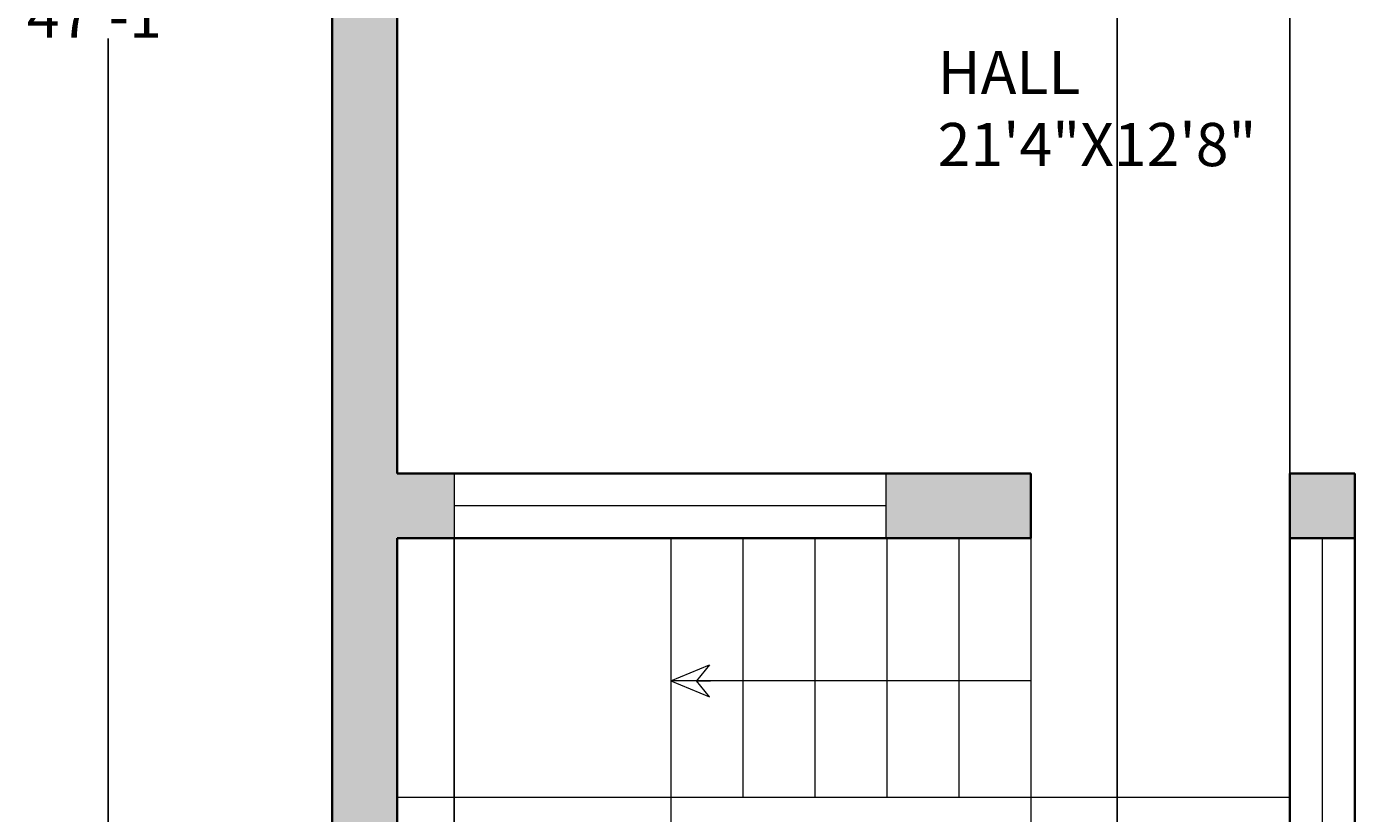
# Model space of a CAD drawing. Units: inches. Extents: x 37 to 706, y -568 to 110.
# Tile 7 of 24: x 37 to 223, y -342 to -233. Entities that reach past the tile are written whole.
import ezdxf

# ---------------------------------------------------------------- set-up
doc = ezdxf.new("R2010")
doc.units = ezdxf.units.IN
doc.header["$MEASUREMENT"] = 0
for name, color, linetype, lineweight in [('A-ANNO-DIMS', 2, 'Continuous', 18), ('A-AREA-IDEN', 7, 'Continuous', 18), ('A-FLOR-STRS', 7, 'Continuous', 18), ('A-GLAZ', 4, 'Continuous', 18), ('A-WALL', 7, 'Continuous', 35), ('A-WALL-PATT', 252, 'Continuous', 13)]:
    doc.layers.add(name, color=color, linetype=linetype, lineweight=lineweight)
doc.styles.get("Standard").update_dxf_attribs({"font": 'arial.ttf'})
doc.dimstyles.get("Standard").update_dxf_attribs({"dimtxt": 0.18, "dimasz": 0.18, "dimexe": 0.18, "dimexo": 0.0625, "dimgap": 0.09, "dimtad": 0, "dimtih": 1, "dimtoh": 1, "dimdec": 0, "dimzin": 0, "dimdsep": 46, "dimlunit": 3, "dimtxsty": 'Standard', "dimcen": 0.09, "dimadec": 0, "dimazin": 0, "dimtfac": 1, "dimtdec": 0, "dimtofl": 0, "dimtmove": 0, "dimatfit": 3, "dimfxl": 1, "dimtolj": 1, "dimtzin": 0, "dimarcsym": 0})

# ---------------------------------------------------------------- blocks, each defined once
blk = doc.blocks.new('*D3')
at = {"layer": 'A-ANNO-DIMS', "color": 0, "lineweight": -2, "transparency": 16777216}
for p, q in [((78.9, 51.29), (47.67, 51.29)), ((47.85, 51.11), (47.85, -228.11)), ((47.85, -513.53), (47.85, -234.31)), ((78.9, -513.71), (47.67, -513.71))]:
    blk.add_line(p, q, dxfattribs=at)
at = {"layer": 'A-ANNO-DIMS', "color": 0, "transparency": 16777216}
for points in [[(47.82, 51.11), (47.88, 51.11), (47.85, 51.29)], [(47.82, -513.53), (47.88, -513.53), (47.85, -513.71)]]:
    blk.add_solid(points, dxfattribs=at)
at = {"layer": 'Defpoints', "color": 0, "transparency": 16777216}
for p in [(78.96, 51.29), (47.85, -513.71), (78.96, -513.71)]:
    blk.add_point(p, dxfattribs=at)
at = {"layer": 'A-ANNO-DIMS', "color": 0, "transparency": 16777216, "insert": (47.85, -231.21), "char_height": 6, "attachment_point": 5}
blk.add_mtext('\\A1;47\'-1"', dxfattribs=at)
blk = doc.blocks.new('WIN-60')
for p, q in [((60, 9), (0, 9)), ((0, 9), (0, 0)), ((60, 0), (60, 9)), ((60, 4.5), (0, 4.5)), ((0, 0), (60, 0))]:
    blk.add_line(p, q)
blk = doc.blocks.new('*D51')
at = {"layer": 'A-ANNO-DIMS', "color": 0, "lineweight": -2, "transparency": 16777216}
for p, q in [((220.96, -294.77), (220.96, -567.64)), ((251.96, -294.77), (251.96, -567.64)), ((221.14, -567.46), (236.13, -567.46)), ((251.78, -567.46), (236.79, -567.46))]:
    blk.add_line(p, q, dxfattribs=at)
at = {"layer": 'A-ANNO-DIMS', "color": 0, "transparency": 16777216}
for points in [[(221.14, -567.43), (221.14, -567.49), (220.96, -567.46)], [(251.78, -567.43), (251.78, -567.49), (251.96, -567.46)]]:
    blk.add_solid(points, dxfattribs=at)
at = {"layer": 'Defpoints', "color": 0, "transparency": 16777216}
for p in [(220.96, -294.71), (251.96, -294.71), (251.96, -567.46)]:
    blk.add_point(p, dxfattribs=at)
at = {"layer": 'A-ANNO-DIMS', "color": 0, "transparency": 16777216, "insert": (236.46, -567.46), "char_height": 0.18, "attachment_point": 5}
blk.add_mtext('\\A1;2\'-7"', dxfattribs=at)
blk = doc.blocks.new('*D54')
at = {"layer": 'A-ANNO-DIMS', "color": 0, "lineweight": -2, "transparency": 16777216}
for p, q in [((87.96, -303.77), (87.96, -567.64)), ((95.87, -303.77), (95.87, -567.64)), ((88.14, -567.46), (91.59, -567.46)), ((95.69, -567.46), (92.24, -567.46))]:
    blk.add_line(p, q, dxfattribs=at)
at = {"layer": 'A-ANNO-DIMS', "color": 0, "transparency": 16777216}
for points in [[(88.14, -567.43), (88.14, -567.49), (87.96, -567.46)], [(95.69, -567.43), (95.69, -567.49), (95.87, -567.46)]]:
    blk.add_solid(points, dxfattribs=at)
at = {"layer": 'Defpoints', "color": 0, "transparency": 16777216}
for p in [(87.96, -303.71), (95.87, -303.71), (95.87, -567.46)]:
    blk.add_point(p, dxfattribs=at)
at = {"layer": 'A-ANNO-DIMS', "color": 0, "transparency": 16777216, "insert": (91.91, -567.46), "char_height": 0.18, "attachment_point": 5}
blk.add_mtext('\\A1;0\'-8"', dxfattribs=at)
blk = doc.blocks.new('*D62')
at = {"layer": 'A-ANNO-DIMS', "color": 0, "lineweight": -2, "transparency": 16777216}
for p, q in [((187.96, -142.77), (187.96, -567.64)), ((211.96, -142.77), (211.96, -567.64)), ((188.14, -567.46), (199.63, -567.46)), ((211.78, -567.46), (200.29, -567.46))]:
    blk.add_line(p, q, dxfattribs=at)
at = {"layer": 'A-ANNO-DIMS', "color": 0, "transparency": 16777216}
for points in [[(188.14, -567.43), (188.14, -567.49), (187.96, -567.46)], [(211.78, -567.43), (211.78, -567.49), (211.96, -567.46)]]:
    blk.add_solid(points, dxfattribs=at)
at = {"layer": 'Defpoints', "color": 0, "transparency": 16777216}
for p in [(187.96, -142.71), (211.96, -142.71), (211.96, -567.46)]:
    blk.add_point(p, dxfattribs=at)
at = {"layer": 'A-ANNO-DIMS', "color": 0, "transparency": 16777216, "insert": (199.96, -567.46), "char_height": 0.18, "attachment_point": 5}
blk.add_mtext('\\A1;2\'-0"', dxfattribs=at)

msp = doc.modelspace()

# ---------------------------------------------------------------- hatches: boundary and pattern name
at = {"layer": 'A-WALL-PATT'}
h = msp.add_hatch(color=256, dxfattribs=at)
h.dxf.hatch_style = 1
h.paths.add_polyline_path([(220.96, -351.71), (211.96, -351.71), (211.96, -513.71), (254.96, -513.71), (254.96, -504.71), (220.96, -504.71)], flags=17)
h.paths.add_polyline_path([(220.96, -294.71), (211.96, -294.71), (211.96, -303.71), (220.96, -303.71)], flags=17)
h.paths.add_polyline_path([(175.96, -294.71), (155.87, -294.71), (155.87, -303.71), (155.96, -303.71), (175.96, -303.71)], flags=17)
h.paths.add_polyline_path([(220.96, -16.71), (211.96, -16.71), (211.96, -142.71), (220.96, -142.71)], flags=17)
h.paths.add_polyline_path([(357.96, 51.29), (78.96, 51.29), (78.96, -513.71), (87.96, -513.71), (87.96, -303.71), (95.87, -303.71), (95.87, -294.71), (87.96, -294.71), (87.96, -142.71), (187.96, -142.71), (187.96, -133.71), (87.96, -133.71), (87.96, -25.71), (106.96, -25.71), (106.96, -16.71), (87.96, -16.71), (87.96, 42.29), (348.96, 42.29), (348.96, 17.13), (348.96, -133.71), (246.96, -133.71), (246.96, -142.71), (348.96, -142.71), (348.96, -294.71), (251.96, -294.71), (251.96, -303.71), (348.96, -303.71), (348.96, -351.71), (260.96, -351.71), (260.96, -329.71), (251.96, -329.71), (251.96, -360.71), (327.45, -360.71), (348.96, -360.71), (348.96, -504.71), (314.96, -504.71), (314.96, -513.71), (357.96, -513.71)])
h.paths.add_polyline_path([(416.96, -303.71), (402.96, -303.71), (402.96, -151.71), (478.96, -151.71), (478.96, -142.71), (402.96, -142.71), (402.96, -22.71), (409.96, -22.71), (409.96, -13.71), (402.96, -13.71), (402.96, 42.29), (663.96, 42.29), (663.96, -303.71), (566.96, -303.71), (566.96, -312.71), (663.96, -312.71), (663.96, -360.71), (575.96, -360.71), (575.96, -338.71), (566.96, -338.71), (566.96, -360.71), (566.96, -369.71), (642.45, -369.71), (663.96, -369.71), (663.96, -513.71), (629.96, -513.71), (629.96, -522.71), (672.96, -522.71), (672.96, 51.29), (393.96, 51.29), (393.96, -522.71), (402.96, -522.71), (402.96, -312.71), (416.96, -312.71)])
h.paths.add_polyline_path([(490.96, -303.71), (476.96, -303.71), (476.96, -312.71), (490.96, -312.71)], flags=17)
h.paths.add_polyline_path([(535.96, -303.71), (526.96, -303.71), (526.96, -312.71), (535.96, -312.71)], flags=17)
h.paths.add_polyline_path([(535.96, -369.71), (526.96, -369.71), (526.96, -522.71), (569.96, -522.71), (569.96, -513.71), (535.96, -513.71)], flags=17)
h.paths.add_polyline_path([(511.96, -13.71), (502.96, -13.71), (502.96, -151.71), (511.96, -151.71)], flags=17)
h.paths.add_polyline_path([(651.54, -142.71), (651.54, -120.18), (642.54, -120.18), (642.54, -142.71), (550.54, -142.71), (550.54, -120.71), (541.54, -120.71), (541.54, -142.71), (537.96, -142.71), (537.96, -151.71), (651.54, -151.71)], flags=17)
h.paths.add_polyline_path([(651.54, -85.71), (541.54, -85.71), (541.54, -94.71), (651.54, -94.71)], flags=17)
h.paths.add_polyline_path([(476.96, -13.71), (469.96, -13.71), (469.96, -22.71), (476.96, -22.71)], flags=17)
h.paths.add_polyline_path([(185.96, -16.71), (166.96, -16.71), (166.96, -25.71), (185.96, -25.71)], flags=17)
h.paths.add_polyline_path([(168.91, -414.72), (214.62, -414.72), (214.62, -392.33), (168.91, -392.33)], flags=25)

# ---------------------------------------------------------------- linework, layer by layer
at = {"layer": 'A-FLOR-STRS'}
for p, q in [((125.96, -303.71), (125.96, -339.71)), ((135.96, -303.71), (135.96, -339.71)), ((145.96, -303.71), (145.96, -339.71)), ((145.96, -303.71), (145.96, -339.71)), ((155.96, -303.71), (155.96, -339.71)), ((165.96, -303.71), (165.96, -339.71)), ((165.96, -303.71), (165.96, -339.71)), ((175.96, -303.71), (175.96, -351.71)), ((125.96, -323.51), (131.33, -321.3)), ((131.33, -321.3), (129.52, -323.51)), ((175.96, -323.51), (125.96, -323.51)), ((125.96, -323.51), (131.33, -325.73)), ((129.52, -323.51), (131.5, -323.51)), ((131.33, -325.73), (129.52, -323.51)), ((125.96, -339.71), (87.96, -339.71)), ((211.96, -339.71), (125.96, -339.71)), ((125.96, -339.71), (125.96, -449.71))]:
    msp.add_line(p, q, dxfattribs=at)
at = {"layer": 'A-GLAZ'}
msp.add_line((216.46, -351.71), (216.46, -303.71), dxfattribs=at)
at = {"layer": 'A-WALL'}
for p, q in [((78.96, 51.29), (78.96, -513.71)), ((87.96, -142.71), (87.96, -294.71)), ((87.96, -294.71), (175.96, -294.71)), ((175.96, -303.71), (175.96, -294.71)), ((211.96, -294.71), (211.96, -513.71)), ((211.96, -294.71), (220.96, -294.71)), ((220.96, -294.71), (220.96, -504.71)), ((87.96, -303.71), (175.96, -303.71)), ((87.96, -303.71), (87.96, -513.71)), ((211.96, -303.71), (220.96, -303.71))]:
    msp.add_line(p, q, dxfattribs=at)

# ---------------------------------------------------------------- block references
at = {"layer": 'A-GLAZ'}
msp.add_blockref('WIN-60', (95.87, -303.71), dxfattribs=at)

# ---------------------------------------------------------------- texts
at = {"layer": 'A-AREA-IDEN', "insert": (163.04, -236.05), "char_height": 6, "attachment_point": 1}
msp.add_mtext('HALL\\P21\'4"X12\'8"', dxfattribs=at)

# ---------------------------------------------------------------- dimensions: what is measured, and where the dimension line sits
at = {"layer": 'A-ANNO-DIMS'}
dim = msp.add_linear_dim(base=(47.85, -513.71), p1=(78.96, 51.29), p2=(78.96, -513.71), angle=90, dimstyle='Standard', override={"dimtxt": 6, "dimclrd": 0, "dimclre": 0, "dimclrt": 0}, dxfattribs=at)
dim.commit()
dim.dimension.update_dxf_attribs({"geometry": '*D3', "text_midpoint": (47.85, -231.21)})
for base, p1, p2, picture, middle in [((211.96, -567.46), (187.96, -142.71), (211.96, -142.71), '*D62', (199.96, -567.46)), ((251.96, -567.46), (220.96, -294.71), (251.96, -294.71), '*D51', (236.46, -567.46)), ((95.87, -567.46), (87.96, -303.71), (95.87, -303.71), '*D54', (91.91, -567.46))]:
    dim = msp.add_linear_dim(base=base, p1=p1, p2=p2, dimstyle='Standard', override={"dimdec": 1, "dimlfac": 1, "dimrnd": 0, "dimzin": 1, "dimdsep": 46, "dimlunit": 4, "dimfrac": 2}, dxfattribs=at)
    dim.commit()
    dim.dimension.update_dxf_attribs({"geometry": picture, "text_midpoint": middle})

doc.saveas('drawing.dxf')
